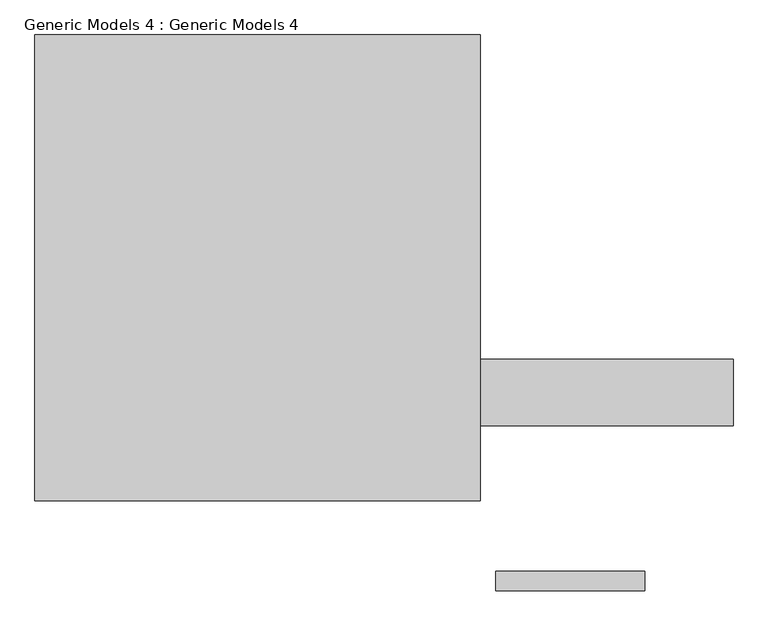
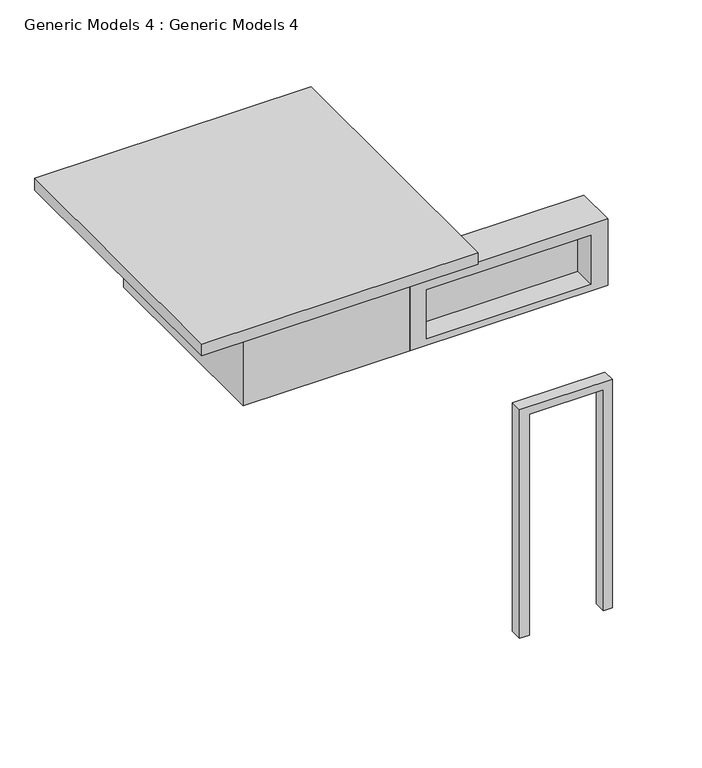
"""IFC4 building model written with IfcOpenShell, lengths in millimetres: proxy geometry, Generic Models 4 : Generic Models 4."""

from ifc_helpers import new_model, si_unit, frame, origin, place, context, project, spatial, polyline, outline, extrude, faceted_brep, source, transform, mapped, element, save


def generic_models_4_generic_models_4_0081fb0e(model_context):
    return source(origin(), model_context, "Body", "SolidModel", [
        extrude(outline(polyline([(-20865.5403308, -5163.8518738), (-14058.3403308, -5163.8518738), (-14058.3403308, -12283.0936073), (-20865.5403308, -12283.0936073), (-20865.5403308, -5163.8518738)])), frame((0.0, 0.0, 8983.2997843), z_axis=(0.0, 0.0, 1.0), x_axis=(1.0, 0.0, 0.0)), (0.0, 0.0, 1.0), 304.8),
        extrude(outline(polyline([(-19189.1403308, -11138.7186143), (-19189.1403308, -6040.1518738), (-15074.3403308, -6040.1518738), (-15074.3403308, -11138.7186143), (-19189.1403308, -11138.7186143)])), frame((0.0, 0.0, 6400.8), z_axis=(0.0, 0.0, 1.0), x_axis=(1.0, 0.0, 0.0)), (0.0, 0.0, 1.0), 2582.4997843),
        faceted_brep([(-15074.3403308, -11138.7186143, 8120.778612), (-10197.5403308, -11138.7186143, 8120.778612), (-10197.5403308, -10116.8518738, 8120.778612), (-15074.3403308, -10116.8518738, 8120.778612), (-15074.3403308, -11138.7186143, 6400.8), (-15074.3403308, -10116.8518738, 6400.8), (-10197.5403308, -10116.8518738, 6400.8), (-10197.5403308, -11138.7186143, 6400.8), (-10616.6403308, -11138.7186143, 7839.4991871), (-10616.6403308, -11138.7186143, 6562.2859637), (-14666.7718866, -11138.7186143, 6562.2859637), (-14666.7718866, -11138.7186143, 7839.4991871), (-10616.6403308, -10579.9186143, 7839.4991871), (-14666.7718866, -10579.9186143, 7839.4991871), (-14666.7718866, -10579.9186143, 6562.2859637), (-10616.6403308, -10579.9186143, 6562.2859637)], [[[0, 1, 2, 3]], [[4, 5, 6, 7]], [[1, 0, 4, 7], [8, 9, 10, 11]], [[2, 1, 7, 6]], [[3, 2, 6, 5]], [[0, 3, 5, 4]], [[12, 13, 14, 15]], [[12, 15, 9, 8]], [[15, 14, 10, 9]], [[14, 13, 11, 10]], [[13, 12, 8, 11]]]),
        extrude(outline(polyline([(0.0, -13827.7509168), (0.0, -13588.4403308), (5747.4569224, -13588.4403308), (5747.4569224, -11759.6403308), (0.0, -11759.6403308), (0.0, -11547.4298818), (5950.6569224, -11547.4298818), (5950.6569224, -13827.7509168), (0.0, -13827.7509168)])), frame((0.0, -13660.1518738, 0.0), z_axis=(0.0, 1.0, 0.0), x_axis=(0.0, 0.0, 1.0)), (0.0, 0.0, 1.0), 304.8),
    ])


if __name__ == "__main__":
    model = new_model("IFC4")
    model_context = context("Model", 3, world=origin())
    ifc_project = project(units=[si_unit("LENGTHUNIT", "METRE", prefix="MILLI")], contexts=[model_context])
    site = spatial("IfcSite", under=ifc_project)
    building = spatial("IfcBuilding", under=site)
    placement = place(None, origin())
    generic_models_4_generic_models_4_shape = generic_models_4_generic_models_4_0081fb0e(model_context)
    element("IfcBuildingElementProxy", 1, Name="Generic Models 4 : Generic Models 4", ObjectType="Generic Models 4 : Generic Models 4", at=placement, inside=building, context=model_context, shape_type="MappedRepresentation", body=[
        mapped(generic_models_4_generic_models_4_shape, transform((0.0, 0.0, 0.0), x_axis=(1.0, 0.0, 0.0), y_axis=(0.0, 1.0, 0.0), z_axis=(0.0, 0.0, 1.0))),
    ])
    save(model, "model.ifc")
